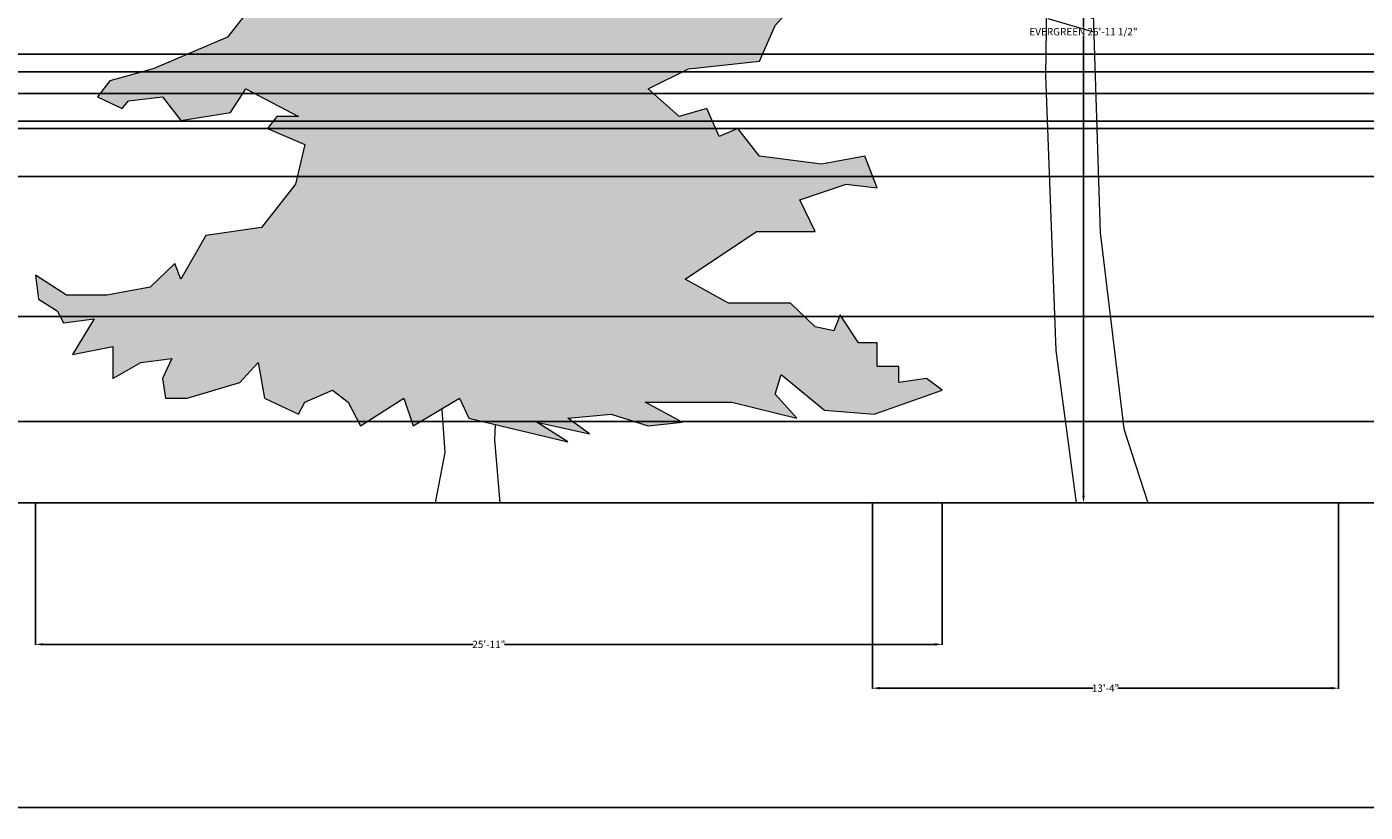
# Model space of a CAD drawing. Units: inches. Extents: x 481 to 2783, y 1975 to 3327.
# Tile 10 of 13: x 1872 to 2331, y 2017 to 2286. Entities that reach past the tile are written whole.
import ezdxf

# ---------------------------------------------------------------- set-up
doc = ezdxf.new("R2010")
doc.units = ezdxf.units.IN
doc.header["$MEASUREMENT"] = 0
for name, color, linetype, lineweight in [('A-ANNO-DIMS', 50, 'Continuous', 18), ('C-TOPO', 7, 'Continuous', 25), ('L-PLNT', 7, 'Continuous', 13)]:
    doc.layers.add(name, color=color, linetype=linetype, lineweight=lineweight)
doc.layers.add('L-PLNT-PATT', color=116, linetype='Continuous', lineweight=13, true_color=0x136734)
doc.styles.get("Standard").update_dxf_attribs({"font": 'arial.ttf'})
doc.dimstyles.get("Standard").update_dxf_attribs({"dimtxt": 2.5, "dimasz": 2.5, "dimexe": 0.18, "dimexo": 0.0625, "dimgap": 0.09, "dimtad": 0, "dimtih": 1, "dimtoh": 1, "dimzin": 0, "dimdsep": 46, "dimlunit": 3, "dimtxsty": 'Standard', "dimcen": 0.09, "dimadec": 0, "dimazin": 0, "dimtfac": 1, "dimtofl": 0, "dimtmove": 0, "dimatfit": 3, "dimfxl": 1, "dimtolj": 1, "dimtzin": 0, "dimarcsym": 0})

# ---------------------------------------------------------------- blocks, each defined once
blk = doc.blocks.new('Tree - evergreen elevation')
for p, q in [((-8.263, 7.598), (-8.747, 14.105)), ((-0.771, 9.56), (-0.69, 11.833)), ((0, 0), (-0.771, 9.56)), ((-9.75, 0), (-8.263, 7.598))]:
    blk.add_line(p, q)
for points in [[(-3.9, 142.35), (-6.596, 132.037), (-10.801, 128.443), (-17.81, 126.047), (-20.614, 122.452), (-17.81, 123.65), (-15.007, 123.051), (-13.605, 118.858), (-16.876, 114.065), (-21.549, 111.07), (-22.951, 109.872), (-19.212, 110.471), (-19.68, 109.273), (-26.222, 105.079), (-34.633, 101.485), (-41.175, 96.693), (-43.511, 93.098), (-41.175, 94.296), (-36.969, 95.494), (-34.633, 94.296), (-32.764, 94.296), (-29.493, 95.494)], [(-3.759, 141.97), (-1.074, 131.643), (2.437, 127.141), (8.84, 124.493), (6.568, 124.493), (4.09, 123.169), (4.296, 121.846), (7.807, 117.874), (16.069, 116.02), (10.492, 115.226), (5.535, 113.372), (6.981, 112.843), (5.948, 110.989), (10.286, 112.048), (6.775, 109.401), (11.732, 108.077), (9.873, 107.282), (13.797, 102.516), (21.852, 101.192), (25.983, 103.84), (28.048, 106.488), (27.842, 105.164), (27.429, 101.457), (24.124, 97.75), (23.091, 93.513), (19.58, 93.513), (23.505, 91.66), (28.255, 90.866), (31.973, 91.925), (29.081, 89.806), (24.537, 88.747), (26.809, 88.218), (22.472, 86.099), (24.95, 85.57), (17.308, 84.246), (21.852, 80.804), (29.081, 79.215), (36.723, 80.009), (39.821, 82.392), (40.028, 80.009), (45.398, 76.567)], [(-29.25, 95.55), (-25.287, 94.296), (-22.016, 94.296), (-23.885, 91.301), (-20.614, 91.301), (-23.418, 87.108), (-35.567, 80.518), (-36.035, 76.924), (-41.175, 70.334), (-52.389, 65.542), (-58.931, 63.744), (-60.8, 61.348), (-57.062, 59.551), (-56.128, 60.749), (-50.987, 61.348), (-48.184, 57.754), (-40.707, 58.952), (-38.371, 62.546), (-30.427, 58.353), (-33.698, 58.353), (-35.1, 56.556), (-29.493, 54.159), (-30.894, 48.169), (-36.035, 41.579), (-44.446, 40.381), (-48.184, 33.791), (-49.118, 36.188), (-52.857, 32.593), (-59.399, 31.395), (-65.473, 31.395), (-70.146, 34.39), (-69.679, 30.796), (-66.875, 28.999), (-65.941, 27.202), (-61.268, 27.801), (-64.539, 22.409), (-58.464, 23.607), (-58.464, 18.815), (-54.258, 21.211), (-49.586, 21.81), (-50.987, 18.815), (-50.52, 15.82), (-47.249, 15.82), (-39.306, 18.216), (-36.502, 21.211), (-35.567, 15.82), (-30.427, 13.423), (-29.493, 15.221), (-25.287, 17.018), (-22.951, 15.221), (-21.081, 11.626), (-14.539, 15.82), (-13.138, 11.626), (-6.128, 15.82), (-4.726, 12.824), (10.226, 9.23), (5.554, 12.225), (13.497, 10.428), (10.226, 12.824), (16.768, 13.423), (22.376, 11.626), (27.516, 12.225), (21.909, 15.221), (34.993, 15.221), (44.806, 12.824), (41.535, 16.419), (42.469, 19.414), (49.011, 14.023), (56.487, 13.423), (66.768, 17.018), (64.431, 18.815), (60.226, 18.216), (60.226, 20.612), (56.955, 20.612), (56.955, 24.206), (54.151, 24.206), (51.348, 28.4), (50.413, 26.004), (47.609, 26.603), (43.871, 30.197), (38.731, 30.197), (34.525, 30.197), (27.983, 33.791), (38.731, 40.98), (47.609, 40.98), (45.273, 45.773), (52.282, 48.169), (56.955, 47.57), (55.086, 52.362), (48.544, 51.164), (39.198, 52.362), (35.927, 56.556), (33.123, 55.357), (31.254, 59.551), (27.049, 58.353), (22.376, 62.546), (28.451, 65.542), (39.198, 66.74), (41.535, 72.131), (45.273, 76.325)]]:
    blk.add_lwpolyline(points)
blk = doc.blocks.new('Tree - palm elevation')
for p, q in [((-5.567, 196.707), (-4.987, 201.167)), ((-4.407, 195.716), (-3.247, 200.672)), ((-7.5, 199.68), (-7.5, 197.946)), ((-2.474, 193.733), (-1.315, 199.433)), ((15.116, 194.477), (17.822, 198.689)), ((18.015, 195.716), (20.914, 198.689)), ((-6.727, 197.202), (-11.366, 197.45)), ((-1.121, 190.759), (0.232, 196.955)), ((9.317, 191.255), (10.283, 196.955)), ((11.829, 192.99), (13.182, 197.45)), ((13.956, 194.229), (14.729, 196.955)), ((19.368, 196.459), (19.948, 193.733)), ((20.914, 196.459), (21.301, 194.972)), ((21.301, 196.459), (22.847, 198.441)), ((22.074, 196.707), (23.427, 195.716)), ((23.234, 196.707), (23.62, 197.698)), ((-3.441, 194.477), (-10.013, 195.716)), ((5.837, 187.786), (7.577, 194.229)), ((16.082, 194.972), (17.822, 192.494)), ((18.015, 195.468), (18.981, 192.494)), ((-25.283, 191.751), (-29.342, 192.246)), ((-20.064, 191.751), (-25.863, 193.238)), ((-21.031, 191.998), (-21.804, 183.325)), ((-15.232, 191.255), (-20.644, 193.981)), ((-9.433, 189.025), (-15.618, 193.238)), ((-1.894, 192.494), (-9.24, 193.733)), ((-0.541, 189.52), (-7.307, 192.494)), ((0.038, 188.281), (1.778, 193.981)), ((11.25, 192.494), (15.889, 190.512)), ((14.536, 193.981), (17.242, 191.255)), ((-29.729, 190.759), (-31.469, 191.255)), ((-30.309, 190.512), (-30.695, 189.025)), ((-28.763, 190.759), (-28.763, 188.281)), ((-26.443, 191.503), (-26.636, 186.051)), ((-23.737, 191.751), (-24.51, 185.06)), ((-17.551, 191.503), (-20.451, 181.343)), ((-14.265, 190.759), (-18.131, 182.086)), ((-11.753, 189.768), (-15.425, 182.83)), ((-6.147, 186.299), (-9.24, 190.264)), ((-5.76, 190.016), (0.618, 185.308)), ((1.005, 185.803), (2.358, 190.759)), ((4.098, 185.06), (4.678, 190.512)), ((8.544, 190.512), (13.763, 189.52)), ((19.368, 187.29), (26.133, 189.768)), ((-8.08, 188.034), (-12.912, 182.83)), ((-5.76, 188.034), (-1.508, 182.582)), ((6.997, 188.529), (12.216, 187.786)), ((9.51, 184.317), (15.502, 188.034)), ((15.695, 186.299), (19.368, 188.777)), ((24.78, 187.538), (31.546, 188.777)), ((-4.987, 185.803), (-10.979, 182.086)), ((-2.668, 185.803), (1.198, 181.343)), ((1.005, 182.582), (2.938, 186.547)), ((4.871, 186.051), (10.09, 186.547)), ((14.536, 185.803), (19.948, 180.847)), ((17.242, 186.547), (23.041, 180.599)), ((20.721, 187.042), (25.167, 181.343)), ((23.814, 187.29), (26.907, 181.343)), ((26.133, 187.29), (29.419, 181.838)), ((28.066, 187.29), (30.966, 182.582)), ((29.806, 186.795), (32.319, 183.078)), ((29.999, 186.795), (33.092, 187.29)), ((32.512, 186.299), (35.218, 186.299)), ((33.479, 186.051), (34.445, 182.83)), ((35.605, 185.556), (37.151, 185.308)), ((-3.247, 183.821), (-8.08, 181.838)), ((2.938, 182.582), (6.61, 183.821)), ((4.871, 181.591), (8.544, 184.812)), ((7.77, 183.325), (16.082, 179.856)), ((11.25, 184.812), (17.628, 180.352)), ((35.798, 185.308), (36.958, 181.591)), ((38.118, 184.317), (38.504, 181.838)), ((-1.315, 181.591), (-5.374, 181.095)), ((5.644, 181.838), (13.569, 178.865)), ((39.857, 182.83), (40.244, 181.591)), ((-15.618, 179.36), (-20.644, 178.617)), ((-15.038, 179.36), (-10.786, 174.404)), ((-12.332, 180.104), (-9.433, 175.643)), ((-10.206, 180.104), (-8.08, 175.891)), ((-8.273, 180.104), (-6.147, 176.635)), ((-6.34, 179.608), (-4.6, 177.13)), ((-4.021, 179.36), (-2.861, 177.378)), ((-0.348, 180.352), (-1.894, 180.104)), ((4.098, 180.847), (8.35, 179.608)), ((7.384, 178.369), (10.476, 179.36)), ((11.829, 177.874), (18.015, 179.113)), ((18.015, 177.13), (26.133, 179.113)), ((-21.031, 177.626), (-24.897, 176.387)), ((-20.064, 177.626), (-15.812, 172.67)), ((-17.358, 178.617), (-13.299, 173.661)), ((-1.701, 176.882), (-8.66, 175.396)), ((-0.928, 176.882), (-1.508, 173.909)), ((1.585, 177.13), (0.038, 174.652)), ((1.585, 177.13), (6.61, 176.139)), ((6.224, 178.121), (8.157, 175.148)), ((8.157, 178.121), (10.476, 172.422)), ((10.476, 177.874), (12.796, 169.696)), ((13.182, 177.874), (14.729, 166.97)), ((15.889, 177.13), (16.855, 164.492)), ((-25.09, 175.148), (-28.376, 174.404)), ((-25.476, 174.652), (-21.224, 167.466)), ((-24.317, 175.891), (-18.711, 168.457)), ((-22.191, 176.635), (-16.391, 169.448)), ((-4.214, 175.148), (-14.072, 170.935)), ((-4.6, 174.9), (-4.021, 166.722)), ((-2.668, 176.387), (-2.376, 170.594)), ((2.551, 175.891), (-0.928, 171.431)), ((2.938, 175.891), (8.737, 173.413)), ((18.981, 175.891), (19.561, 163.005)), ((20.914, 175.891), (30.966, 176.635)), ((21.688, 175.396), (22.074, 161.518)), ((-27.409, 173.413), (-30.695, 172.67)), ((-27.989, 172.422), (-26.056, 166.227)), ((-26.829, 173.661), (-23.544, 167.218)), ((-6.92, 172.917), (-5.374, 163.253)), ((3.711, 174.404), (-0.541, 167.961)), ((4.291, 173.909), (12.216, 168.953)), ((23.814, 174.404), (25.554, 160.279)), ((25.554, 173.661), (33.285, 173.661)), ((26.52, 173.165), (28.066, 159.784)), ((-28.956, 172.174), (-32.435, 170.192)), ((-29.922, 170.687), (-27.989, 165.235)), ((-8.466, 171.678), (-16.585, 167.713)), ((-8.853, 170.935), (-7.113, 160.527)), ((5.257, 171.926), (-0.155, 163.005)), ((6.417, 170.439), (14.729, 164.492)), ((28.839, 172.174), (36.378, 170.687)), ((29.226, 171.926), (30.966, 158.545)), ((30.966, 170.687), (38.891, 167.713)), ((-32.628, 167.961), (-33.208, 167.961)), ((-31.082, 169.944), (-32.435, 169.2)), ((-31.662, 168.705), (-31.082, 165.483)), ((-12.139, 167.961), (-19.098, 162.014)), ((-10.979, 168.457), (-7.887, 157.801)), ((7.384, 168.705), (0.812, 157.553)), ((32.126, 169.696), (32.512, 158.545)), ((34.058, 168.705), (34.445, 158.545)), ((-32.628, 167.713), (-32.435, 165.979)), ((-12.719, 166.722), (-9.046, 154.828)), ((8.544, 165.979), (16.662, 160.527)), ((35.412, 167.713), (41.404, 164.988)), ((36.378, 166.474), (35.605, 158.792)), ((-14.265, 164.244), (-19.678, 158.049)), ((-14.265, 163.749), (-10.786, 154.828)), ((9.317, 164.244), (2.358, 154.332)), ((37.731, 165.235), (36.958, 159.288)), ((37.924, 165.235), (41.404, 163.749)), ((38.504, 164.492), (38.504, 159.536)), ((10.09, 162.51), (17.435, 157.058)), ((39.664, 163.253), (42.37, 161.766)), ((39.857, 162.757), (39.857, 160.031)), ((40.824, 161.766), (41.21, 160.031)), ((41.21, 161.518), (42.757, 160.279)), ((-16.005, 160.031), (-19.484, 154.084)), ((-15.618, 160.775), (-12.332, 154.332)), ((10.863, 159.784), (4.484, 152.35)), ((-16.585, 158.545), (-13.106, 152.35)), ((11.443, 157.553), (16.855, 154.332)), ((-17.358, 155.819), (-14.845, 151.358)), ((11.829, 155.075), (6.804, 150.119)), ((-18.131, 153.589), (-19.484, 151.606)), ((12.216, 153.093), (16.082, 151.606)), ((-17.938, 152.597), (-16.972, 151.111)), ((12.603, 151.111), (8.544, 148.385)), ((12.603, 149.872), (15.116, 149.128)), ((12.216, 148.137), (10.09, 147.393)), ((12.409, 146.898), (13.763, 146.402)), ((12.409, 145.659), (11.056, 145.659)), ((-4.081, 140.645), (0.753, 138.261)), ((-4.081, 137.547), (0.753, 135.163)), ((-4.081, 129.205), (1.124, 126.821)), ((-4.081, 127.298), (1.31, 123.246)), ((-4.081, 121.578), (1.31, 120.863)), ((-4.267, 114.428), (1.682, 108.708)), ((-4.453, 112.283), (1.682, 105.133)), ((-4.639, 102.273), (1.868, 100.604)), ((-4.453, 99.651), (2.24, 98.459)), ((-4.453, 91.071), (2.426, 89.641)), ((-4.825, 83.921), (2.612, 81.061)), ((-4.639, 81.299), (2.797, 78.916)), ((-4.639, 78.916), (2.797, 76.771))]:
    blk.add_line(p, q)
for points in [[(-2.363, 170.553), (-3.88, 148.505), (-4.988, 69.634), (-3.325, 24.869), (0, 0)], [(-0.116, 162.848), (0.554, 143.532), (2.217, 96.635), (3.88, 44.054), (7.76, 12.079), (11.64, 0)]]:
    blk.add_lwpolyline(points)
for centre, radius, start, end in [((-18.427, 181.448), 19.715, 350.285, 64.11229), ((25.595, 171.567), 25.395, 91.40319, 163.882), ((-21.738, 166.094), 25.899, 27.67115, 112.5305), ((23.687, 155.341), 32.188, 56.19272, 134.3213), ((-9.259, 151.732), 28.386, 68.38311, 147.5322), ((14.394, 148.393), 32.752, 113.7592, 177.4133), ((5.828, 132.718), 45.639, 35.98777, 95.82273), ((-32.8, 147.923), 45.309, 356.1943, 41.37848)]:
    blk.add_arc(centre, radius, start, end)
blk = doc.blocks.new('*D56')
at = {"layer": 'A-ANNO-DIMS', "color": 0, "lineweight": -2, "transparency": 16777216}
for p, q in [((2321.97, 2546.55), (2385.65, 2546.55)), ((2385.47, 2544.05), (2385.47, 2336.07)), ((2385.47, 2125.32), (2385.47, 2333.3)), ((2321.97, 2122.82), (2385.65, 2122.82))]:
    blk.add_line(p, q, dxfattribs=at)
at = {"layer": 'A-ANNO-DIMS', "color": 0, "transparency": 16777216}
for points in [[(2385.05, 2544.05), (2385.89, 2544.05), (2385.47, 2546.55)], [(2385.05, 2125.32), (2385.89, 2125.32), (2385.47, 2122.82)]]:
    blk.add_solid(points, dxfattribs=at)
at = {"layer": 'Defpoints', "color": 0, "transparency": 16777216}
for p in [(2321.91, 2546.55), (2385.47, 2546.55), (2321.91, 2122.82)]:
    blk.add_point(p, dxfattribs=at)
at = {"layer": 'A-ANNO-DIMS', "color": 0, "transparency": 16777216, "insert": (2385.47, 2334.69), "char_height": 2.5, "attachment_point": 5}
blk.add_mtext('\\A1;PALM 35\'-3 1/2"', dxfattribs=at)
blk = doc.blocks.new('*D57')
at = {"layer": 'A-ANNO-DIMS', "color": 0, "lineweight": -2, "transparency": 16777216}
for p, q in [((2161.9, 2122.76), (2161.9, 2059.08)), ((2321.91, 2122.76), (2321.91, 2059.08)), ((2164.4, 2059.26), (2237.64, 2059.26)), ((2319.41, 2059.26), (2246.17, 2059.26))]:
    blk.add_line(p, q, dxfattribs=at)
at = {"layer": 'A-ANNO-DIMS', "color": 0, "transparency": 16777216}
for points in [[(2164.4, 2059.68), (2164.4, 2058.84), (2161.9, 2059.26)], [(2319.41, 2059.68), (2319.41, 2058.84), (2321.91, 2059.26)]]:
    blk.add_solid(points, dxfattribs=at)
at = {"layer": 'Defpoints', "color": 0, "transparency": 16777216}
for p in [(2161.9, 2122.82), (2321.91, 2122.82), (2321.91, 2059.26)]:
    blk.add_point(p, dxfattribs=at)
at = {"layer": 'A-ANNO-DIMS', "color": 0, "transparency": 16777216, "insert": (2241.9, 2059.26), "char_height": 2.5, "attachment_point": 5}
blk.add_mtext('\\A1;13\'-4"', dxfattribs=at)
blk = doc.blocks.new('*D62')
at = {"layer": 'A-ANNO-DIMS', "color": 0, "lineweight": -2, "transparency": 16777216}
for p, q in [((2185.87, 2446.33), (2234.51, 2446.33)), ((2234.33, 2443.83), (2234.33, 2285.96)), ((2234.33, 2125.32), (2234.33, 2283.19)), ((2185.87, 2122.82), (2234.51, 2122.82))]:
    blk.add_line(p, q, dxfattribs=at)
at = {"layer": 'A-ANNO-DIMS', "color": 0, "transparency": 16777216}
for points in [[(2233.91, 2443.83), (2234.75, 2443.83), (2234.33, 2446.33)], [(2233.91, 2125.32), (2234.75, 2125.32), (2234.33, 2122.82)]]:
    blk.add_solid(points, dxfattribs=at)
at = {"layer": 'Defpoints', "color": 0, "transparency": 16777216}
for p in [(2185.8, 2446.33), (2234.33, 2446.33), (2185.8, 2122.82)]:
    blk.add_point(p, dxfattribs=at)
at = {"layer": 'A-ANNO-DIMS', "color": 0, "transparency": 16777216, "insert": (2234.33, 2284.57), "char_height": 2.5, "attachment_point": 5}
blk.add_mtext('\\A1;EVERGREEN 26\'-11 1/2"', dxfattribs=at)
blk = doc.blocks.new('*D63')
at = {"layer": 'A-ANNO-DIMS', "color": 0, "lineweight": -2, "transparency": 16777216}
for p, q in [((1874.65, 2122.76), (1874.65, 2074.11)), ((2185.8, 2122.76), (2185.8, 2074.11)), ((1877.15, 2074.29), (2024.85, 2074.29)), ((2183.3, 2074.29), (2035.6, 2074.29))]:
    blk.add_line(p, q, dxfattribs=at)
at = {"layer": 'A-ANNO-DIMS', "color": 0, "transparency": 16777216}
for points in [[(1877.15, 2074.71), (1877.15, 2073.88), (1874.65, 2074.29)], [(2183.3, 2074.71), (2183.3, 2073.88), (2185.8, 2074.29)]]:
    blk.add_solid(points, dxfattribs=at)
at = {"layer": 'Defpoints', "color": 0, "transparency": 16777216}
for p in [(1874.65, 2122.82), (2185.8, 2122.82), (2185.8, 2074.29)]:
    blk.add_point(p, dxfattribs=at)
at = {"layer": 'A-ANNO-DIMS', "color": 0, "transparency": 16777216, "insert": (2030.23, 2074.29), "char_height": 2.5, "attachment_point": 5}
blk.add_mtext('\\A1;25\'-11"', dxfattribs=at)
blk = doc.blocks.new('*D66')
at = {"layer": 'A-ANNO-DIMS', "color": 0, "lineweight": -2, "transparency": 16777216}
for p, q in [((591.06, 2122.76), (591.06, 2018.14)), ((2669.26, 2122.76), (2669.26, 2018.14)), ((593.56, 2018.32), (1624.92, 2018.32)), ((2666.76, 2018.32), (1635.4, 2018.32))]:
    blk.add_line(p, q, dxfattribs=at)
at = {"layer": 'A-ANNO-DIMS', "color": 0, "transparency": 16777216}
for points in [[(593.56, 2018.74), (593.56, 2017.9), (591.06, 2018.32)], [(2666.76, 2018.74), (2666.76, 2017.9), (2669.26, 2018.32)]]:
    blk.add_solid(points, dxfattribs=at)
at = {"layer": 'Defpoints', "color": 0, "transparency": 16777216}
for p in [(591.06, 2122.82), (2669.26, 2122.82), (2669.26, 2018.32)]:
    blk.add_point(p, dxfattribs=at)
at = {"layer": 'A-ANNO-DIMS', "color": 0, "transparency": 16777216, "insert": (1630.16, 2018.32), "char_height": 2.5, "attachment_point": 5}
blk.add_mtext('\\A1;173\'-2"', dxfattribs=at)
blk = doc.blocks.new('*D70')
at = {"layer": 'A-ANNO-DIMS', "color": 0, "lineweight": -2, "transparency": 16777216}
for p, q in [((1794.5, 2150.82), (2773.94, 2150.82)), ((2773.76, 2148.32), (2773.76, 2138.17)), ((2773.76, 2125.32), (2773.76, 2135.48)), ((1794.5, 2122.82), (2773.94, 2122.82))]:
    blk.add_line(p, q, dxfattribs=at)
at = {"layer": 'A-ANNO-DIMS', "color": 0, "transparency": 16777216}
for points in [[(2773.34, 2148.32), (2774.17, 2148.32), (2773.76, 2150.82)], [(2773.34, 2125.32), (2774.17, 2125.32), (2773.76, 2122.82)]]:
    blk.add_solid(points, dxfattribs=at)
at = {"layer": 'Defpoints', "color": 0, "transparency": 16777216}
for p in [(1794.44, 2150.82), (2773.76, 2150.82), (1794.44, 2122.82)]:
    blk.add_point(p, dxfattribs=at)
at = {"layer": 'A-ANNO-DIMS', "color": 0, "transparency": 16777216, "insert": (2773.76, 2136.82), "char_height": 2.5, "attachment_point": 5}
blk.add_mtext('\\A1;2\'-4"', dxfattribs=at)
blk = doc.blocks.new('*D71')
at = {"layer": 'A-ANNO-DIMS', "color": 0, "lineweight": -2, "transparency": 16777216}
for p, q in [((1737.9, 2186.82), (2773.94, 2186.82)), ((2773.76, 2184.32), (2773.76, 2170.19)), ((2773.76, 2153.32), (2773.76, 2167.45)), ((1794.5, 2150.82), (2773.94, 2150.82))]:
    blk.add_line(p, q, dxfattribs=at)
at = {"layer": 'A-ANNO-DIMS', "color": 0, "transparency": 16777216}
for points in [[(2773.34, 2184.32), (2774.17, 2184.32), (2773.76, 2186.82)], [(2773.34, 2153.32), (2774.17, 2153.32), (2773.76, 2150.82)]]:
    blk.add_solid(points, dxfattribs=at)
at = {"layer": 'Defpoints', "color": 0, "transparency": 16777216}
for p in [(1737.84, 2186.82), (2773.76, 2186.82), (1794.44, 2150.82)]:
    blk.add_point(p, dxfattribs=at)
at = {"layer": 'A-ANNO-DIMS', "color": 0, "transparency": 16777216, "insert": (2773.76, 2168.82), "char_height": 2.5, "attachment_point": 5}
blk.add_mtext('\\A1;3\'-0"', dxfattribs=at)
blk = doc.blocks.new('*D72')
at = {"layer": 'A-ANNO-DIMS', "color": 0, "lineweight": -2, "transparency": 16777216}
for p, q in [((1737.9, 2234.82), (2773.94, 2234.82)), ((2773.76, 2232.32), (2773.76, 2212.19)), ((2773.76, 2189.32), (2773.76, 2209.45)), ((1737.9, 2186.82), (2773.94, 2186.82))]:
    blk.add_line(p, q, dxfattribs=at)
at = {"layer": 'A-ANNO-DIMS', "color": 0, "transparency": 16777216}
for points in [[(2773.34, 2232.32), (2774.17, 2232.32), (2773.76, 2234.82)], [(2773.34, 2189.32), (2774.17, 2189.32), (2773.76, 2186.82)]]:
    blk.add_solid(points, dxfattribs=at)
at = {"layer": 'Defpoints', "color": 0, "transparency": 16777216}
for p in [(1737.84, 2234.82), (2773.76, 2234.82), (1737.84, 2186.82)]:
    blk.add_point(p, dxfattribs=at)
at = {"layer": 'A-ANNO-DIMS', "color": 0, "transparency": 16777216, "insert": (2773.76, 2210.82), "char_height": 2.5, "attachment_point": 5}
blk.add_mtext('\\A1;4\'-0"', dxfattribs=at)
blk = doc.blocks.new('*D74')
at = {"layer": 'A-ANNO-DIMS', "color": 0, "lineweight": -2, "transparency": 16777216}
for p, q in [((1412.86, 2270.82), (2773.94, 2270.82)), ((2773.76, 2268.32), (2773.76, 2263.69)), ((2773.76, 2256.32), (2773.76, 2260.95)), ((1417, 2253.82), (2773.94, 2253.82))]:
    blk.add_line(p, q, dxfattribs=at)
at = {"layer": 'A-ANNO-DIMS', "color": 0, "transparency": 16777216}
for points in [[(2773.34, 2268.32), (2774.17, 2268.32), (2773.76, 2270.82)], [(2773.34, 2256.32), (2774.17, 2256.32), (2773.76, 2253.82)]]:
    blk.add_solid(points, dxfattribs=at)
at = {"layer": 'Defpoints', "color": 0, "transparency": 16777216}
for p in [(1412.79, 2270.82), (2773.76, 2270.82), (1416.94, 2253.82)]:
    blk.add_point(p, dxfattribs=at)
at = {"layer": 'A-ANNO-DIMS', "color": 0, "transparency": 16777216, "insert": (2773.76, 2262.32), "char_height": 2.5, "attachment_point": 5}
blk.add_mtext('\\A1;1\'-5"', dxfattribs=at)
blk = doc.blocks.new('*D75')
at = {"layer": 'A-ANNO-DIMS', "color": 0, "lineweight": -2, "transparency": 16777216}
for p, q in [((2773.76, 2276.82), (2773.76, 2279.32)), ((2773.76, 2279.32), (2776.26, 2279.32)), ((1794.5, 2276.82), (2773.94, 2276.82)), ((2773.76, 2273.32), (2773.76, 2274.32)), ((1794.5, 2270.82), (2773.94, 2270.82))]:
    blk.add_line(p, q, dxfattribs=at)
at = {"layer": 'A-ANNO-DIMS', "color": 0, "transparency": 16777216}
for points in [[(2773.34, 2274.32), (2774.17, 2274.32), (2773.76, 2276.82)], [(2773.34, 2273.32), (2774.17, 2273.32), (2773.76, 2270.82)]]:
    blk.add_solid(points, dxfattribs=at)
at = {"layer": 'Defpoints', "color": 0, "transparency": 16777216}
for p in [(1794.44, 2276.82), (2773.76, 2276.82), (1794.44, 2270.82)]:
    blk.add_point(p, dxfattribs=at)
at = {"layer": 'A-ANNO-DIMS', "color": 0, "transparency": 16777216, "insert": (2779.67, 2279.32), "char_height": 2.5, "attachment_point": 5}
blk.add_mtext('\\A1;0\'-6"', dxfattribs=at)
blk = doc.blocks.new('*D82')
at = {"layer": 'A-ANNO-DIMS', "color": 0, "lineweight": -2, "transparency": 16777216}
for p, q in [((1785.5, 2263.36), (2773.94, 2263.36)), ((2773.76, 2260.86), (2773.76, 2258.72)), ((2773.76, 2253.86), (2773.76, 2255.99)), ((1785.5, 2251.36), (2773.94, 2251.36))]:
    blk.add_line(p, q, dxfattribs=at)
at = {"layer": 'A-ANNO-DIMS', "color": 0, "transparency": 16777216}
for points in [[(2773.34, 2260.86), (2774.17, 2260.86), (2773.76, 2263.36)], [(2773.34, 2253.86), (2774.17, 2253.86), (2773.76, 2251.36)]]:
    blk.add_solid(points, dxfattribs=at)
at = {"layer": 'Defpoints', "color": 0, "transparency": 16777216}
for p in [(1785.44, 2263.36), (1785.44, 2251.36), (2773.76, 2251.36)]:
    blk.add_point(p, dxfattribs=at)
at = {"layer": 'A-ANNO-DIMS', "color": 0, "transparency": 16777216, "insert": (2773.76, 2257.36), "char_height": 2.5, "attachment_point": 5}
blk.add_mtext('\\A1;1\'-0"', dxfattribs=at)

msp = doc.modelspace()

# ---------------------------------------------------------------- hatches: boundary and pattern name
at = {"layer": 'L-PLNT-PATT'}
h = msp.add_hatch(color=256, dxfattribs=at)
h.set_gradient(color1=(88, 186, 72), color2=(19, 155, 72))
h.paths.add_polyline_path([(2073.399, 2314.279), (2090.767, 2317.288), (2085.135, 2318.49), (2094.991, 2323.306), (2089.828, 2324.508), (2100.155, 2326.915), (2106.727, 2331.73), (2098.278, 2329.324), (2087.483, 2331.128), (2078.563, 2335.339), (2086.542, 2335.339), (2088.89, 2344.968), (2096.401, 2353.393), (2097.339, 2361.817), (2097.807, 2364.826), (2093.114, 2358.808), (2083.726, 2352.791), (2065.42, 2355.8), (2056.503, 2366.631), (2060.727, 2368.438), (2049.462, 2371.446), (2057.441, 2377.462), (2047.583, 2375.055), (2049.93, 2379.269), (2046.644, 2380.471), (2057.909, 2384.684), (2070.584, 2386.489), (2051.807, 2390.702), (2043.828, 2399.729), (2043.36, 2402.736), (2048.992, 2405.745), (2054.155, 2405.745), (2039.603, 2411.763), (2031.624, 2421.994), (2025.25, 2446.511), (2019.075, 2422.889), (2009.519, 2414.722), (1993.59, 2409.276), (1987.217, 2401.106), (1993.59, 2403.829), (1999.96, 2402.468), (2003.146, 2392.939), (1995.712, 2382.046), (1985.093, 2375.239), (1981.906, 2372.517), (1990.404, 2373.878), (1989.34, 2371.156), (1974.473, 2361.624), (1955.358, 2353.456), (1940.49, 2342.566), (1935.182, 2334.396), (1940.49, 2337.119), (1950.049, 2339.841), (1955.358, 2337.119), (1959.605, 2337.119), (1967.481, 2340.003), (1976.598, 2337.119), (1984.031, 2337.119), (1979.784, 2330.312), (1987.217, 2330.312), (1980.845, 2320.783), (1953.235, 2305.807), (1952.172, 2297.639), (1940.49, 2282.662), (1915.005, 2271.772), (1900.138, 2267.686), (1895.89, 2262.241), (1904.385, 2258.157), (1906.508, 2260.879), (1918.191, 2262.241), (1924.562, 2254.073), (1941.554, 2256.796), (1946.863, 2264.963), (1964.916, 2255.434), (1957.483, 2255.434), (1954.296, 2251.35), (1967.039, 2245.903), (1963.855, 2232.29), (1952.172, 2217.313), (1933.057, 2214.591), (1924.562, 2199.614), (1922.439, 2205.062), (1913.942, 2196.892), (1899.074, 2194.169), (1885.27, 2194.169), (1874.651, 2200.976), (1875.712, 2192.808), (1882.084, 2188.724), (1884.207, 2184.64), (1894.827, 2186.001), (1887.393, 2173.748), (1901.199, 2176.47), (1901.199, 2165.58), (1910.758, 2171.025), (1921.375, 2172.386), (1918.191, 2165.58), (1919.253, 2158.773), (1926.686, 2158.773), (1944.738, 2164.218), (1951.11, 2171.025), (1953.235, 2158.773), (1964.916, 2153.326), (1967.039, 2157.412), (1976.598, 2161.496), (1981.906, 2157.412), (1986.156, 2149.242), (2001.024, 2158.773), (2004.208, 2149.242), (2020.139, 2158.773), (2023.325, 2151.965), (2057.305, 2143.797), (2046.687, 2150.603), (2064.738, 2146.519), (2057.305, 2151.965), (2072.172, 2153.326), (2084.917, 2149.242), (2096.598, 2150.603), (2083.856, 2157.412), (2113.591, 2157.412), (2135.892, 2151.965), (2128.458, 2160.135), (2130.581, 2166.941), (2145.448, 2154.689), (2162.438, 2153.326), (2185.803, 2161.496), (2180.492, 2165.58), (2170.935, 2164.218), (2170.935, 2169.664), (2163.502, 2169.664), (2163.502, 2177.831), (2157.129, 2177.831), (2150.759, 2187.363), (2148.634, 2181.918), (2142.262, 2183.279), (2133.767, 2191.447), (2122.086, 2191.447), (2112.527, 2191.447), (2097.66, 2199.614), (2122.086, 2215.952), (2142.262, 2215.952), (2136.953, 2226.845), (2152.882, 2232.29), (2163.502, 2230.929), (2159.254, 2241.819), (2144.387, 2239.096), (2123.147, 2241.819), (2115.713, 2251.35), (2109.341, 2248.625), (2105.093, 2258.157), (2095.537, 2255.434), (2084.917, 2264.963), (2098.723, 2271.772), (2123.147, 2274.495), (2128.458, 2286.746), (2137.368, 2296.744), (2125.033, 2304.65), (2124.563, 2310.066), (2117.522, 2304.65), (2100.155, 2302.845), (2083.726, 2306.457)])
h.paths.add_polyline_path([(726.446, 2320.727), (718.597, 2319.609), (709.875, 2314.018), (699.409, 2308.428), (698.537, 2312.9), (690.688, 2296.128), (704.642, 2299.483), (713.364, 2293.892), (710.747, 2280.475), (695.049, 2274.884), (688.071, 2279.357), (685.455, 2272.648), (679.35, 2271.53), (674.117, 2264.821), (668.011, 2256.995), (675.861, 2250.286), (681.094, 2253.64), (675.177, 2243.917), (679.476, 2244.418), (678.855, 2235.617), (664.523, 2216.742), (647.08, 2215.624), (639.23, 2211.152), (626.148, 2196.616), (631.381, 2187.671), (663.651, 2188.789), (669.756, 2184.317), (684.583, 2191.026), (695.049, 2168.663), (699.409, 2168.663), (719.469, 2193.262), (725.574, 2196.616), (729.935, 2191.026), (729.935, 2183.199), (736.912, 2180.963), (746.506, 2180.963), (749.995, 2188.789), (761.333, 2194.38), (772.671, 2195.498), (777.904, 2199.971), (778.776, 2201.089), (781.392, 2206.679), (784.881, 2204.443), (787.498, 2195.498), (793.603, 2198.852), (795.347, 2196.616), (797.091, 2191.026), (803.197, 2201.089), (809.302, 2201.089), (811.918, 2196.616), (809.302, 2192.144), (816.279, 2194.38), (818.895, 2191.026), (825, 2195.498), (831.106, 2193.262), (843.316, 2180.963), (848.549, 2178.726), (852.91, 2174.254), (889.54, 2177.608), (896.518, 2170.9), (901.751, 2173.136), (887.796, 2191.026), (886.924, 2197.734), (891.285, 2204.443), (883.435, 2225.687), (879.075, 2225.687), (870.353, 2256.995), (861.631, 2258.112), (866.864, 2262.585), (873.841, 2280.475), (859.887, 2295.01), (842.444, 2300.601), (850.293, 2312.9), (843.316, 2334.144), (838.955, 2334.144), (830.233, 2353.152), (825, 2352.034), (818.895, 2352.034), (814.534, 2360.979), (817.151, 2373.278), (824.128, 2373.278), (811.046, 2388.932), (809.286, 2401.34), (802.324, 2409.058), (796.219, 2402.35), (792.731, 2404.586), (791.858, 2410.176), (787.498, 2412.413), (781.392, 2406.822), (774.415, 2407.94), (769.182, 2397.877), (769.182, 2388.932), (776.16, 2385.578), (770.926, 2382.223), (765.694, 2386.696), (750.867, 2372.16), (750.867, 2368.806), (744.762, 2365.452), (746.506, 2362.097), (750.867, 2355.389), (743.017, 2349.798), (735.168, 2355.389), (730.807, 2354.271), (729.063, 2349.798), (735.168, 2348.68), (736.04, 2339.735), (729.221, 2340.853), (721.213, 2333.026), (729.935, 2331.908)])

# ---------------------------------------------------------------- linework, layer by layer
at = {"layer": 'C-TOPO'}
msp.add_line((1794.438, 2122.821), (2669.257, 2122.821), dxfattribs=at)
at = {"layer": 'L-PLNT'}
for p, q in [((2011.907, 2122.821), (2034.065, 2122.821)), ((2231.847, 2122.821), (2256.365, 2122.821))]:
    msp.add_line(p, q, dxfattribs=at)

# ---------------------------------------------------------------- block references
for name, p, xscale, yscale, zscale in [('Tree - palm elevation', (2231.847, 2122.821), 2.106372464461094, 2.106372464461094, 2.106372464461094), ('Tree - evergreen elevation', (2034.065, 2122.821), 2.272610793994812, 2.272610793994812, 2.272610793994812)]:
    msp.add_blockref(name, p, dxfattribs=dict(at, xscale=xscale, yscale=yscale, zscale=zscale))

# ---------------------------------------------------------------- dimensions: what is measured, and where the dimension line sits
at = {"layer": 'A-ANNO-DIMS'}
for base, p1, p2, text, picture, middle in [((2385.469, 2546.553), (2321.909, 2122.821), (2321.909, 2546.553), 'PALM <>', '*D56', (2385.469, 2334.687)), ((2234.329, 2446.327), (2185.803, 2122.821), (2185.803, 2446.327), 'EVERGREEN <>', '*D62', (2234.329, 2284.574))]:
    dim = msp.add_linear_dim(base=base, p1=p1, p2=p2, angle=90, text=text, dimstyle='Standard', override={"dimdec": 1, "dimlfac": 1, "dimrnd": 0, "dimzin": 1, "dimdsep": 46, "dimlunit": 4, "dimfrac": 2}, dxfattribs=at)
    dim.commit()
    dim.dimension.update_dxf_attribs({"geometry": picture, "text_midpoint": middle})
for base, p1, p2, picture, middle in [((2773.757, 2276.821), (1794.438, 2270.821), (1794.438, 2276.821), '*D75', (2779.67, 2279.321)), ((2773.757, 2270.821), (1416.938, 2253.821), (1412.793, 2270.821), '*D74', (2773.757, 2262.321)), ((2773.757, 2251.356), (1785.438, 2263.356), (1785.438, 2251.356), '*D82', (2773.757, 2257.356)), ((2773.757, 2234.821), (1737.842, 2186.821), (1737.842, 2234.821), '*D72', (2773.757, 2210.821)), ((2773.757, 2186.821), (1794.438, 2150.821), (1737.842, 2186.821), '*D71', (2773.757, 2168.821)), ((2773.757, 2150.821), (1794.438, 2122.821), (1794.438, 2150.821), '*D70', (2773.757, 2136.821))]:
    dim = msp.add_linear_dim(base=base, p1=p1, p2=p2, angle=90, dimstyle='Standard', override={"dimdec": 1, "dimlfac": 1, "dimrnd": 0, "dimzin": 1, "dimdsep": 46, "dimlunit": 4, "dimfrac": 2}, dxfattribs=at)
    dim.commit()
    dim.dimension.update_dxf_attribs({"geometry": picture, "text_midpoint": middle})
for base, p1, p2, picture, middle in [((2669.257, 2018.321), (591.063, 2122.821), (2669.257, 2122.821), '*D66', (1630.16, 2018.321)), ((2185.803, 2074.295), (1874.651, 2122.821), (2185.803, 2122.821), '*D63', (2030.227, 2074.295)), ((2321.909, 2059.261), (2161.899, 2122.821), (2321.909, 2122.821), '*D57', (2241.904, 2059.261))]:
    dim = msp.add_linear_dim(base=base, p1=p1, p2=p2, dimstyle='Standard', override={"dimdec": 1, "dimlfac": 1, "dimrnd": 0, "dimzin": 1, "dimdsep": 46, "dimlunit": 4, "dimfrac": 2}, dxfattribs=at)
    dim.commit()
    dim.dimension.update_dxf_attribs({"geometry": picture, "text_midpoint": middle})

doc.saveas('drawing.dxf')
